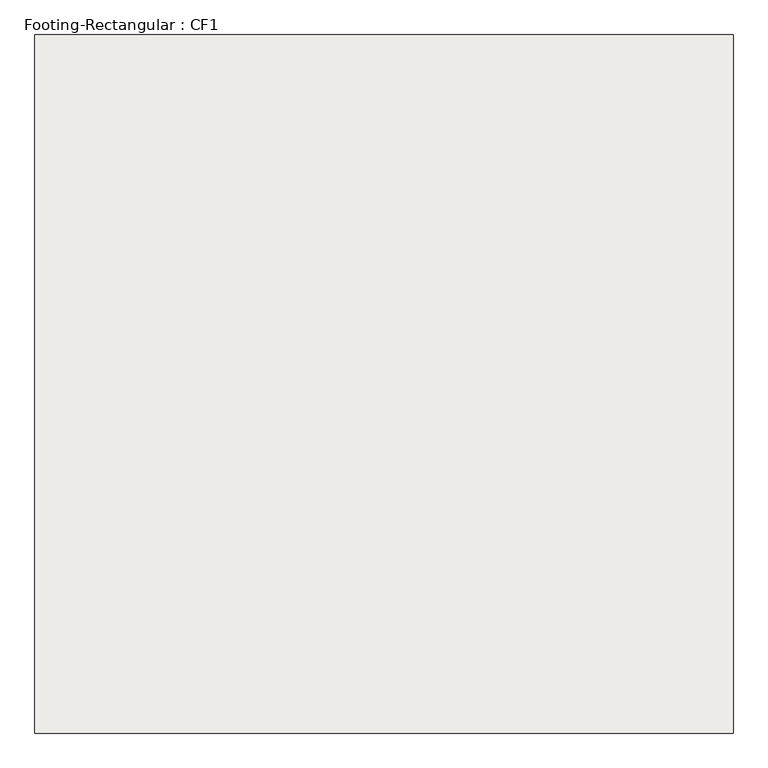
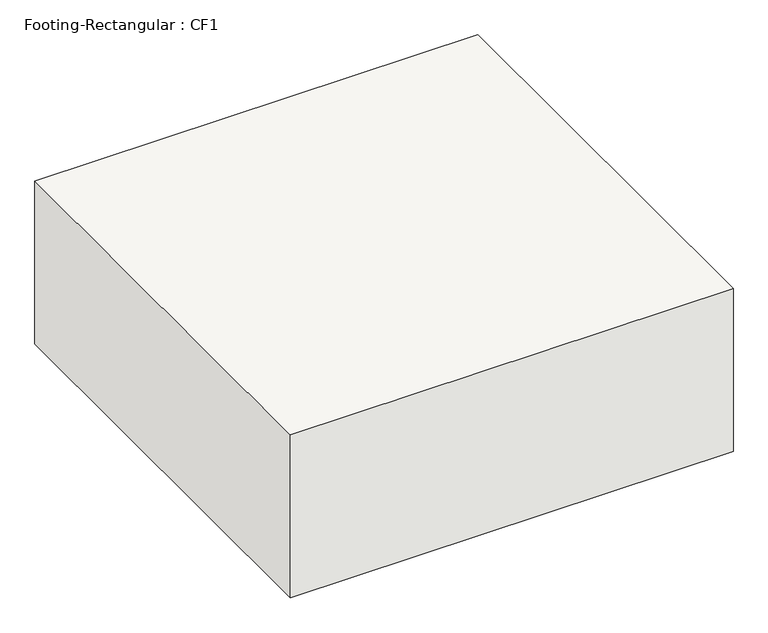
"""IFC4 building model written with IfcOpenShell, lengths in millimetres: slab geometry, Footing-Rectangular : CF1."""

from ifc_helpers import new_model, si_unit, frame, origin, place, context, project, spatial, polyline, outline, extrude, source, transform, mapped, element, save


def footing_rectangular_cf1_e8ad81a8(model_context):
    return source(origin(), model_context, "Body", "SweptSolid", [
        extrude(outline(polyline([(685.8, 685.8), (685.8, -685.8), (-685.8, -685.8), (-685.8, 685.8), (685.8, 685.8)])), frame((0.0, 0.0, -533.4), z_axis=(0.0, 0.0, 1.0), x_axis=(1.0, 0.0, 0.0)), (0.0, 0.0, 1.0), 533.4),
    ])


if __name__ == "__main__":
    model = new_model("IFC4")
    model_context = context("Model", 3, world=origin())
    ifc_project = project(units=[si_unit("LENGTHUNIT", "METRE", prefix="MILLI")], contexts=[model_context])
    site = spatial("IfcSite", under=ifc_project)
    building = spatial("IfcBuilding", under=site)
    placement = place(None, origin())
    footing_rectangular_cf1_shape = footing_rectangular_cf1_e8ad81a8(model_context)
    element("IfcSlab", 1, ObjectType="Footing-Rectangular : CF1", at=placement, inside=building, context=model_context, shape_type="MappedRepresentation", body=[
        mapped(footing_rectangular_cf1_shape, transform((0.0, 0.0, 0.0), x_axis=(1.0, 0.0, 0.0), y_axis=(0.0, 1.0, 0.0), z_axis=(0.0, 0.0, 1.0))),
    ])
    save(model, "model.ifc")

# Revit data of these elements
# Type "Footing-Rectangular : CF1"
#   Width = 1371.6 mm
#   Length = 1371.6 mm
#   Foundation Thickness = 533.4 mm
#   Structural Material [instance default] = Concrete - Cast-in-Place Concrete
#   Assembly Code = ""
# Element 1 (IfcSlab, "Footing-Rectangular : CF1")
#   Materials on its faces: "Concrete - Cast-in-Place Concrete"
# Materials
#   "Concrete - Cast-in-Place Concrete": class "Concrete", colour RGB 192 192 192, transparency 0, Cost = 0
